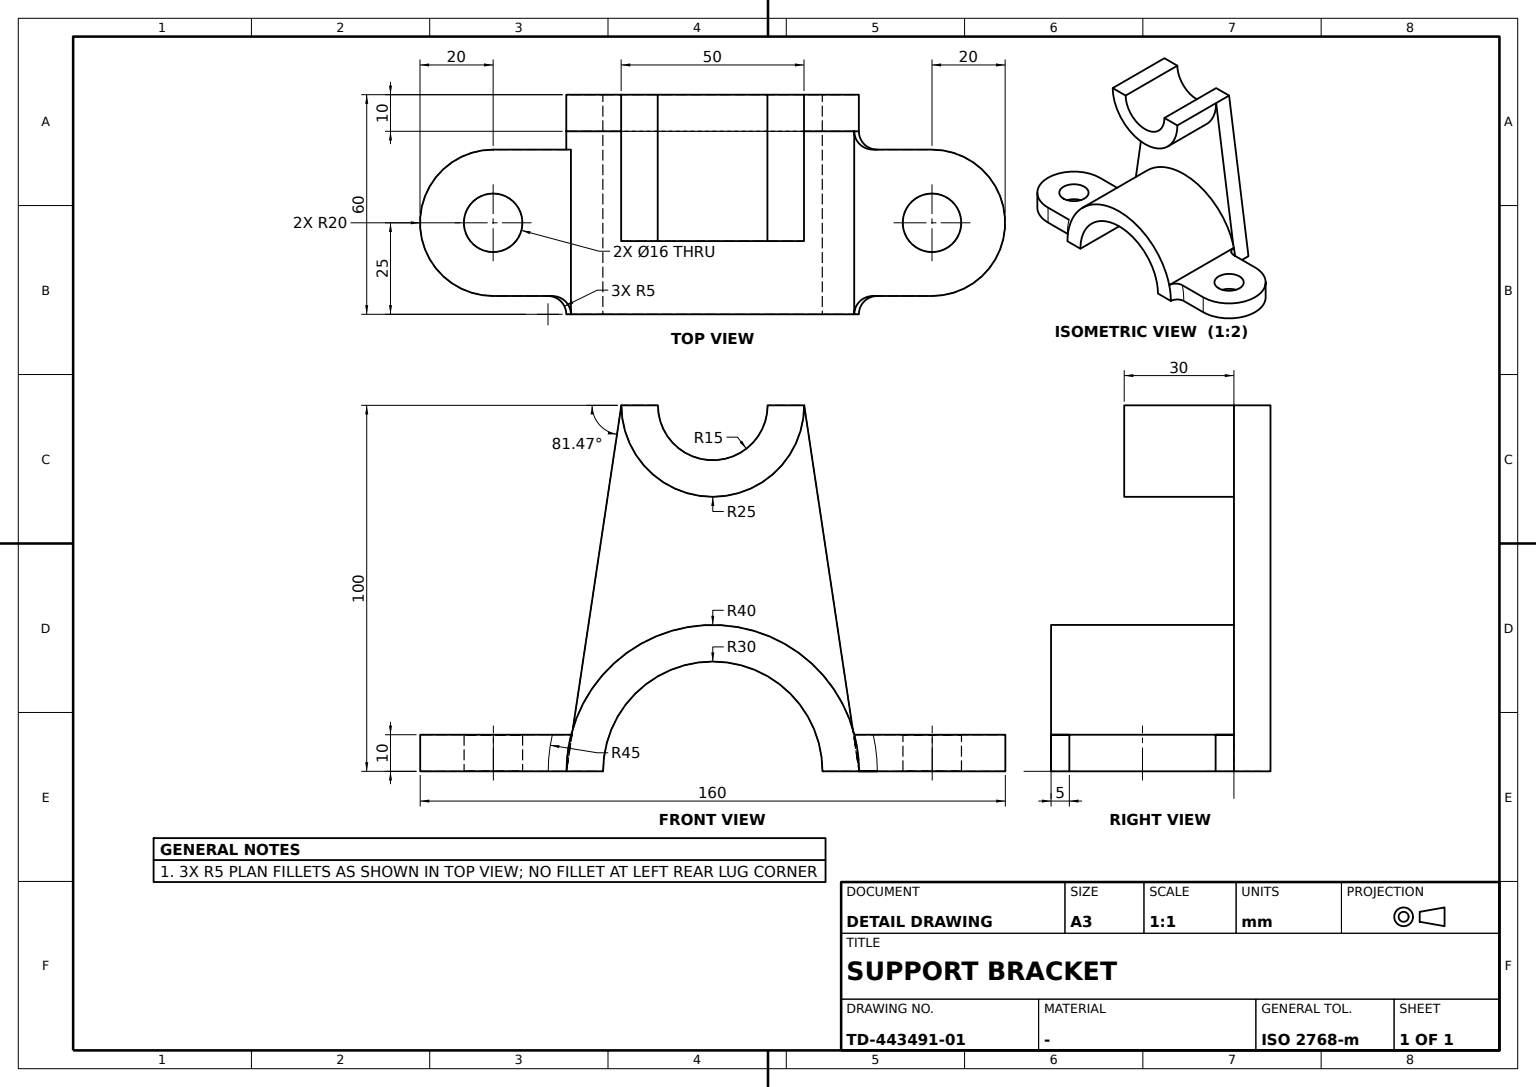
CATIA V5 part; units mm, degrees
sketch "Sketch1" plane through (0, 0, 0) normal (-1, 0, 0) x (0, -1, 0)
  arc A0 (40, 0) -> (-40, 0) centre (0, 0) ccw
  arc A1 (30, 0) -> (-30, 0) centre (0, 0) ccw
  point P0 (-30, 0)
  point P1 (30, 0)
  point P2 (-40, 0)
  point P3 (40, 0)
  point P4 (-40, 0)
  line L0 (-40, 0) -> (-30, 0)
  point P5 (-30, 0)
  point P6 (30, 0)
  line L1 (30, 0) -> (40, 0)
  point P7 (40, 0)
  dimension "radius A0" = 40
  dimension "radius A1" = 30
  constraint coincidence P4 x-axis
  constraint coincidence P4 P2
  constraint coincidence P0 P5
  constraint coincidence P6 x-axis
  constraint coincidence P1 P6
  constraint coincidence P3 P7
  constraint horizontal L0 x-axis
  constraint horizontal L1 x-axis
extrude "Pad1" add sketch "Sketch1" along normal mid plane 50
sketch "Sketch2" plane through (-25, 0, 0) normal (-1, 0, 0) x (0, -1, 0)
  point P0 (-40, 0)
  line L0 (30, 0) -> (40, 0)
  point P1 (40, 0)
  arc A0 (30, 0) -> (-30, 0) centre (0, 0) ccw
  line L1 (-40, 0) -> (-30, 0)
  point P2 (-40, 0)
  point P3 (-40, 0)
  line L2 (-40, 0) -> (-25, 100)
  point P4 (-25, 100)
  line L3 (-25, 100) -> (-15, 100)
  point P5 (25, 100)
  line L4 (25, 100) -> (40, 0)
  point P6 (40, 0)
  arc A1 (-15, 100) -> (15, 100) centre (0, 100) ccw
  point P7 (0, 100)
  point P8 (15, 100)
  line L5 (15, 100) -> (25, 100)
  dimension "radius A1" = 15
  dimension "distance P4 P5" = 50
  dimension "distance origin L3" = 100
  constraint coincidence P0 x-axis
  constraint coincidence P0 P2
  constraint coincidence P3 x-axis
  constraint coincidence P6 x-axis
  constraint coincidence P7 y-axis
  constraint coincidence P7 L3
  constraint coincidence L3 P8
  constraint coincidence L3 L5
  constraint coincidence P6 P1
  constraint horizontal L3 x-axis
  constraint horizontal L5 x-axis
  constraint symmetry L2 L4 y-axis
extrude "Pad2" add sketch "Sketch2" along normal blind 10
sketch "Sketch3" plane through (-25, 0, 0) normal (1, 0, 0) x (0, 1, 0)
  arc A0 (-25, 100) -> (25, 100) centre (0, 100) ccw
  point P0 (0, 100)
  line L0 (25, 100) -> (15, 100) construction
  arc A1 (-15, 100) -> (15, 100) centre (0, 100) ccw construction
  line L1 (-25, 100) -> (-15, 100)
  arc A2 (-15, 100) -> (15, 100) centre (0, 100) ccw
  line L2 (15, 100) -> (25, 100)
  dimension "radius A0" = 25
  constraint coincidence P0 L0
  constraint coincidence L1 L2
  constraint concentricity A0 A1
  constraint horizontal L1 x-axis
  constraint horizontal L2 x-axis
extrude "Pad3" add sketch "Sketch3" along normal blind 30
sketch "Sketch4" plane through (0, 0, 0) normal (0, 0, 1) x (1, 0, 0)
  line L0 (-20, 38) -> (20, 38)
  line L1 (20, 38) -> (20, 60)
  arc A0 (20, 60) -> (-20, 60) centre (0, 60) ccw
  point P0 (0, 60)
  line L2 (-20, 60) -> (-20, 38)
  line L3 (25, -40) -> (25, 40) construction
  circle A1 centre (0, 60) radius 8
  dimension "length L1" = 22
  dimension "length L0" = 40
  dimension "distance L3 L1" = 5
  dimension "radius A0" = 20
  dimension "D5" = 60
  dimension "radius A1" = 8
  dimension "D7" = 38
  constraint horizontal L0 x-axis
  constraint vertical L1 y-axis
  constraint vertical L2 y-axis
extrude "Pad4" add sketch "Sketch4" along normal blind 10
mirror "Mirror1" about plane through (0, 0, 0) normal (0, 1, 0) of "Pad4"
fillet "Fillet1" radius 5 2 edges at (20, 39.6812, 5.0402) (-20, 39.6812, 5.0402)
fillet "Fillet2" radius 5 1 edges at (20, -39.6812, 5.0402)
